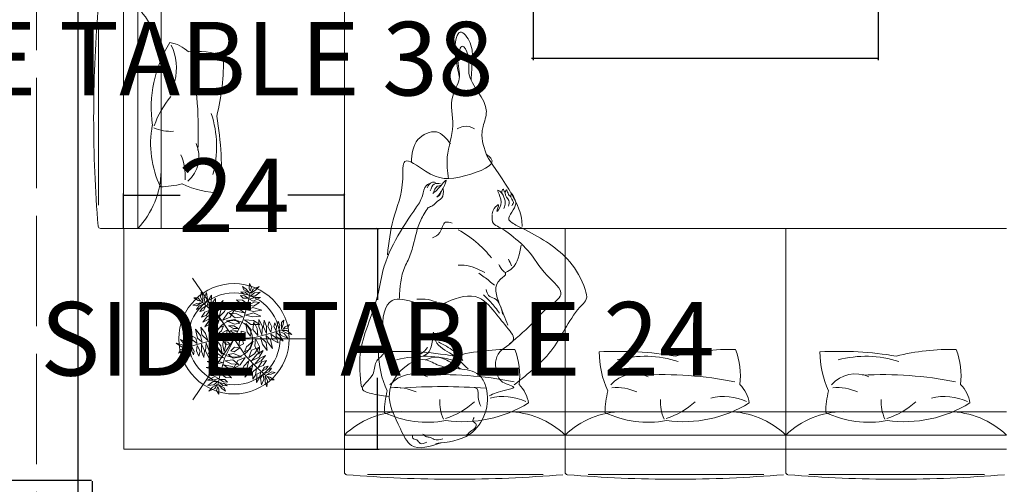
# Model space of a CAD drawing. Units: inches. Extents: x -48 to 50072, y 0 to 21068.
# Tile 48 of 75: x 16 to 123, y 687 to 738. Entities that reach past the tile are written whole.
import ezdxf

# ---------------------------------------------------------------- set-up
doc = ezdxf.new("R2010")
doc.units = ezdxf.units.IN
doc.header["$MEASUREMENT"] = 0
doc.linetypes.add('ACAD_ISO02W100', pattern=[15, 12, -3])
for name, color, linetype, lineweight in [('A-ANNO-DIMS', 2, 'Continuous', 18), ('A-ENTG', 8, 'Continuous', 13), ('C-PROP', 7, 'Continuous', 25), ('C-PROP-REF', 32, 'ACAD_ISO02W100', 13), ('FURNITURE', 44, 'Continuous', 18)]:
    doc.layers.add(name, color=color, linetype=linetype, lineweight=lineweight)
doc.styles.get("Standard").update_dxf_attribs({"font": 'arial.ttf'})
doc.dimstyles.get("Standard").update_dxf_attribs({"dimtxt": 8, "dimasz": 0.18, "dimexe": 0.18, "dimexo": 0.0625, "dimgap": 0.09, "dimtad": 0, "dimtih": 1, "dimtoh": 1, "dimdec": 1, "dimzin": 0, "dimdsep": 46, "dimlunit": 4, "dimtxsty": 'Standard', "dimblk": 'ARCHTICK', "dimcen": 0.09, "dimadec": 0, "dimazin": 0, "dimtfac": 1, "dimtdec": 1, "dimtofl": 0, "dimtmove": 0, "dimatfit": 3, "dimldrblk": 'ARCHTICK', "dimfxl": 1, "dimtolj": 1, "dimtzin": 0, "dimarcsym": 0})

# ---------------------------------------------------------------- blocks, each defined once
blk = doc.blocks.new('SIDE TABLE 2X2')
at = {"layer": 'FURNITURE'}
for q in [(622.06, 188.07), (609.55, 181.47), (622.04, 174.85)]:
    blk.add_line((617.55, 181.47), q, dxfattribs=at)
blk.add_lwpolyline([(605.55, 169.47), (629.55, 169.47), (629.55, 193.47), (605.55, 193.47)], close=True, dxfattribs=at)
for radius in [6, 5, 2]:
    blk.add_circle((617.55, 181.47), radius, dxfattribs=at)
blk = doc.blocks.new('DFGS')
at = {"layer": 'FURNITURE'}
for centre, radius, start, end in [((-6087.14, 813.36), 9.64, 104.9394, 132.5633), ((-6112.38, 805.26), 28.66, 21.6133, 37.4184), ((-6094.33, 816.04), 4.48, 81.3108, 116.3418), ((-6080.05, 821.2), 16.31, 184.0297, 223.6176), ((-6099.45, 813.66), 7.12, 22.214, 60.8038), ((-6126.91, 783.89), 49.66, 32.8076, 46.9), ((-6094.76, 804.41), 13.97, 20.7975, 53.8819), ((-6116.99, 784.16), 44.49, 32.4999, 45.375), ((-6080.96, 813.35), 11.17, 174.5959, 197.1556), ((-6092.61, 815.13), 5.43, 281.6061, 309.1892), ((-6087.9, 807.73), 4.17, 346.5527, 60.4145), ((-6080.21, 815.37), 12.85, 204.9913, 241.6537), ((-6089.91, 803.33), 6.58, 30.5945, 59.6065), ((-6086.56, 817.99), 12.2, 280.9279, 305.5545), ((-6095.16, 815.51), 14.47, 307.7029, 318.9387)]:
    blk.add_arc(centre, radius, start, end, dxfattribs=at)
blk = doc.blocks.new('3+2 seater sofa')
at = {"layer": 'FURNITURE', "ltscale": 3}
for p, q in [((1464.23, 851.06), (1464.23, 827.06)), ((1484.15, 839.06), (1484.15, 851.06)), ((1484.15, 839.06), (1484.15, 827.06)), ((1392.23, 827.06), (1416.23, 827.06)), ((1416.23, 827.06), (1440.23, 827.06)), ((1440.23, 827.06), (1464.23, 827.06)), ((1404.23, 807.13), (1392.23, 807.13)), ((1404.23, 807.13), (1416.23, 807.13)), ((1428.23, 807.13), (1416.23, 807.13)), ((1428.23, 807.13), (1440.23, 807.13)), ((1452.23, 807.13), (1440.23, 807.13)), ((1452.23, 807.13), (1464.23, 807.13))]:
    blk.add_line(p, q, dxfattribs=at)
at = {"layer": 'FURNITURE'}
for p, q in [((1486.69, 839.06), (1486.69, 851.06)), ((1488.23, 827.03, 0), (1488.23, 851.06)), ((1490.98, 848.68), (1490.98, 839.06)), ((1484.15, 844.83), (1484.15, 839.06)), ((1484.15, 833.29), (1484.15, 839.06)), ((1484.15, 839.06, 0), (1484.15, 827.06)), ((1486.69, 839.06), (1486.69, 827.06)), ((1490.98, 829.57), (1490.98, 839.06)), ((1416.23, 800.54), (1416.23, 827.06)), ((1440.23, 800.54), (1440.23, 827.06)), ((1464.23, 800.54), (1464.23, 827.06)), ((1490.74, 827.06), (1464.23, 827.06)), ((1484.13, 827.06), (1490.75, 827.06)), ((1398.46, 807.13), (1404.23, 807.13)), ((1410, 807.13), (1404.23, 807.13)), ((1404.23, 807.13, 0), (1416.23, 807.13)), ((1416.23, 807.16), (1416.23, 800.53)), ((1422.46, 807.13), (1428.23, 807.13)), ((1434, 807.13), (1428.23, 807.13)), ((1428.23, 807.13, 0), (1440.23, 807.13)), ((1440.23, 807.16), (1440.23, 800.53)), ((1446.46, 807.13), (1452.23, 807.13)), ((1458, 807.13), (1452.23, 807.13)), ((1452.23, 807.13, 0), (1464.23, 807.13)), ((1464.23, 807.16), (1464.23, 800.53)), ((1404.23, 804.59), (1392.23, 804.59)), ((1404.23, 804.59), (1416.23, 804.59)), ((1428.23, 804.59), (1416.23, 804.59)), ((1428.23, 804.59), (1440.23, 804.59)), ((1452.23, 804.59), (1440.23, 804.59)), ((1452.23, 804.59), (1464.23, 804.59)), ((1416.26, 803.06, 0), (1392.23, 803.06)), ((1440.26, 803.06, 0), (1416.23, 803.06)), ((1464.26, 803.06, 0), (1440.23, 803.06)), ((1394.6, 800.3), (1404.23, 800.3)), ((1413.72, 800.3), (1404.23, 800.3)), ((1418.6, 800.3), (1428.23, 800.3)), ((1437.72, 800.3), (1428.23, 800.3)), ((1442.6, 800.3), (1452.23, 800.3)), ((1461.72, 800.3), (1452.23, 800.3))]:
    blk.add_line(p, q, dxfattribs=at)
for centre, radius, start, end in [((1493.43, 844.68), 9.28, 136.5598, 179.0844), ((1348.3, 838.96), 143.19, 0.0378, 4.7508), ((1348.3, 839.15), 143.19, 355.2492, 359.9622), ((1493.43, 833.43), 9.28, 180.9156, 223.4402), ((1490.74, 827.31), 0.255, 270, 355.4933), ((1398.61, 797.86), 9.28, 90.9156, 133.4402), ((1409.85, 797.86), 9.28, 46.5598, 89.0844), ((1422.61, 797.86), 9.28, 90.9156, 133.4402), ((1433.85, 797.86), 9.28, 46.5598, 89.0844), ((1446.61, 797.86), 9.28, 90.9156, 133.4402), ((1457.85, 797.86), 9.28, 46.5598, 89.0844), ((1404.32, 942.98), 143.19, 265.2492, 269.9622), ((1404.13, 942.98), 143.19, 270.0378, 274.7508), ((1415.97, 800.54), 0.255, 274.5067, 0), ((1428.32, 942.98), 143.19, 265.2492, 269.9622), ((1428.13, 942.98), 143.19, 270.0378, 274.7508), ((1439.97, 800.54), 0.255, 274.5067, 0), ((1452.32, 942.98), 143.19, 265.2492, 269.9622), ((1452.13, 942.98), 143.19, 270.0378, 274.7508), ((1463.97, 800.54), 0.255, 274.5067, 0)]:
    blk.add_arc(centre, radius, start, end, dxfattribs=at)
at = {"layer": 'FURNITURE', "yscale": 0.8336162403020807, "zscale": 0.8336162403020807}
for p, xscale, rotation in [((-2239.7, -2678.91), -0.8336162403020807, 35.78436137719967), ((4922.38, 4530.98), 0.8336162403020807, 54.21563862280032), ((4946.38, 4530.98), 0.8336162403020807, 54.21563862280032), ((4970.38, 4530.98), 0.8336162403020807, 54.21563862280032)]:
    blk.add_blockref('DFGS', p, dxfattribs=dict(at, xscale=xscale, rotation=rotation))
blk = doc.blocks.new('Women')
for p, q in [((543.24, 3443.84, -275.77), (543.24, 3443.84, -275.77)), ((536.73, 3442.75, -275.77), (536.73, 3442.75, -275.77)), ((543.24, 3442.75, -275.77), (543.24, 3442.75, -275.77)), ((544.33, 3443.3, -275.77), (544.33, 3443.3, -275.77))]:
    blk.add_line(p, q)
at = {"ltscale": 3}
for centre, radius, start, end in [((540.53, 3448.44, -275.77), 1.62, 79.5148, 123.0894), ((540.33, 3447.37, -275.77), 2.71, 63.6392, 79.5148)]:
    blk.add_arc(centre, radius, start, end, dxfattribs=at)
for start, end in [(90.0228, 94.419), (85.6266, 90.0228)]:
    blk.add_arc((543.1, 3361, -303.2), 60.76, start, end)
for points, knots in [([(540, 3455.11, -275.77), (539.96, 3455.83, -275.77), (539.88, 3457.2, -275.77), (539.79, 3458.92, -275.77), (541.38, 3461.08, -275.77), (541.88, 3458.63, -275.77), (541.63, 3457.17, -275.77), (541.42, 3456.09, -275.77), (541.3, 3455.47, -275.77)], [0, 0, 0, 0, 46.697433, 88.465151, 123.324676, 161.835136, 191.877979, 232.626852, 232.626852, 232.626852, 232.626852]), ([(538.22, 3446.72, -275.77), (538.57, 3447.63, -275.77), (538.99, 3448.73, -275.77), (538.63, 3450.39, -275.77), (537.75, 3452.65, -275.77), (540.77, 3455.04, -275.77), (540.02, 3457.37, -275.77), (541.02, 3459.34, -275.77), (541.69, 3456.94, -275.77), (540.9, 3455.37, -275.77), (542.5, 3452.99, -275.77), (541.62, 3450.02, -275.77), (542.8, 3447.11, -275.77), (542.57, 3445.15, -275.77), (542.48, 3444.36, -275.77)], [0, 0, 0, 0, 60.970115, 74.178445, 111.267097, 210.963126, 255.074467, 279.515708, 307.41666, 359.287359, 403.554034, 473.492101, 549.720465, 601.59141, 601.59141, 601.59141, 601.59141]), ([(546.5, 3446.13, -275.77), (546.43, 3447.04, -275.77), (546.31, 3448.71, -275.77), (543.66, 3449.95, -275.77), (542.7, 3448.73, -275.77), (542.24, 3448.14, -275.77)], [0, 0, 0, 0, 56.575903, 104.225618, 148.354052, 148.354052, 148.354052, 148.354052]), ([(534.44, 3439.16, -275.77), (534.48, 3439.74, -275.77), (534.64, 3442.24, -275.77), (539.62, 3448.28, -275.77), (537.06, 3445.84, -275.77), (541.78, 3444.17, -275.77), (544.01, 3444.26, -275.77), (547.6, 3447.18, -275.77), (547.23, 3443, -275.77), (548.63, 3440.29, -275.77), (548.95, 3437.41, -275.77), (549.1, 3436.09, -275.77)], [0, 0, 0, 0, 42.167956, 184.846032, 188.510605, 261.118314, 357.582537, 412.070511, 453.838275, 554.467695, 638.871943, 638.871943, 638.871943, 638.871943]), ([(543.72, 3442.36, -275.77), (543.51, 3442.61, -275.77), (543.15, 3443.06, -275.77), (542.48, 3444.55, -275.77), (543.22, 3443.72, -275.77), (543.57, 3443.25, -275.77), (543.96, 3442.94, -275.77), (544.17, 3442.76, -275.77)], [0, 0, 0, 0, 25.892768, 46.183307, 59.392839, 73.451861, 90.844376, 90.844376, 90.844376, 90.844376]), ([(544.44, 3443.03, -275.77), (544.34, 3443.34, -275.77), (544.17, 3443.92, -275.77), (543.58, 3443.85, -275.77), (543.32, 3443.82, -275.77)], [0, 0, 0, 0, 18.54008, 34.34859, 34.34859, 34.34859, 34.34859]), ([(544.09, 3442.81, -275.77), (544.04, 3443, -275.77), (543.96, 3443.29, -275.77), (543.74, 3443.48, -275.77), (543.68, 3443.54, -275.77)], [0, 0, 0, 0, 12.899473, 18.839157, 18.839157, 18.839157, 18.839157]), ([(544.78, 3443.38, -275.77), (544.64, 3443.64, -275.77), (544.43, 3444.03, -275.77), (544.02, 3443.98, -275.77), (543.88, 3443.96, -275.77)], [0, 0, 0, 0, 16.968689, 25.728505, 25.728505, 25.728505, 25.728505]), ([(545.63, 3441.73, -275.77), (545.51, 3441.98, -275.77), (545.23, 3442.59, -275.77), (545.09, 3443.61, -275.77), (544.49, 3443.87, -275.77), (544.28, 3443.96, -275.77)], [0, 0, 0, 0, 18.740722, 44.970985, 59.745283, 59.745283, 59.745283, 59.745283]), ([(534.98, 3439.25, -275.77), (535.18, 3439.35, -275.77), (535.5, 3439.52, -275.77), (536.1, 3439.99, -275.77), (535.52, 3440.79, -275.77), (534.94, 3441.7, -275.77), (535.37, 3442.42, -275.77), (535.62, 3442.83, -275.77)], [0, 0, 0, 0, 14.897426, 24.638003, 44.249327, 65.81281, 94.158391, 94.158391, 94.158391, 94.158391]), ([(535.62, 3442.83, -275.77), (535.68, 3442.61, -275.77), (535.76, 3442.25, -275.77), (535.3, 3441.87, -275.77), (535.47, 3441.58, -275.77), (535.57, 3441.42, -275.77)], [0, 0, 0, 0, 13.770952, 22.047872, 32.93541, 32.93541, 32.93541, 32.93541]), ([(535.94, 3441.37, -275.77), (535.88, 3441.59, -275.77), (535.73, 3442.14, -275.77), (536.5, 3442.52, -275.77), (536.12, 3443.33, -275.77), (536, 3442.68, -275.77), (535.8, 3442.49, -275.77), (535.69, 3442.39, -275.77)], [0, 0, 0, 0, 13.81853, 34.349896, 42.048978, 50.626809, 61.603847, 61.603847, 61.603847, 61.603847]), ([(537.72, 3440.56, -275.77), (537.68, 3440.74, -275.77), (537.61, 3441.1, -275.77), (536.74, 3441.86, -275.77), (537.48, 3440.4, -275.77), (536.19, 3441.86, -275.77), (537.47, 3443.4, -275.77), (536.74, 3442.92, -275.77), (536.46, 3442.5, -275.77), (536.22, 3441.82, -275.77), (536.37, 3441.34, -275.77), (536.43, 3441.13, -275.77)], [0, 0, 0, 0, 13.622009, 27.045047, 42.301032, 59.74223, 94.71225, 98.491569, 110.440566, 128.701216, 142.844466, 142.844466, 142.844466, 142.844466]), ([(536.38, 3442.9, -275.77), (536.42, 3443.07, -275.77), (536.51, 3443.43, -275.77), (536.75, 3442.89, -275.77), (536.62, 3442.75, -275.77), (536.58, 3442.71, -275.77)], [0, 0, 0, 0, 7.980072, 16.932683, 20.710806, 20.710806, 20.710806, 20.710806]), ([(544.68, 3441.23, -275.77), (544.5, 3441.29, -275.77), (544.1, 3441.43, -275.77), (543.66, 3441.99, -275.77), (542.92, 3442.25, -275.77), (543.07, 3443.67, -275.77), (543.28, 3442.74, -275.77), (543.51, 3442.48, -275.77), (543.65, 3442.4, -275.77), (543.72, 3442.36, -275.77)], [0, 0, 0, 0, 12.228513, 27.193094, 45.006155, 62.152179, 75.922416, 81.425571, 86.507745, 86.507745, 86.507745, 86.507745]), ([(547.8, 3431.37, -275.77), (547.74, 3432.56, -275.77), (547.67, 3434.02, -275.77), (546.69, 3435.75, -275.77), (546.17, 3437.46, -275.77), (545.78, 3439.51, -275.77), (544.97, 3440.78, -275.77), (544.68, 3441.23, -275.77)], [0, 0, 0, 0, 76.228588, 93.60718, 130.36676, 193.495034, 228.582316, 228.582316, 228.582316, 228.582316]), ([(551.94, 3421.7, -275.77), (552.07, 3422.91, -275.77), (552.43, 3426.3, -275.77), (550.26, 3430.29, -275.77), (549.45, 3436.2, -275.77), (547.26, 3439.37, -275.77), (545.63, 3441.73, -275.77)], [0, 0, 0, 0, 78.836785, 220.670789, 284.620897, 468.343596, 468.343596, 468.343596, 468.343596]), ([(535.98, 3438.49, -275.77), (536.29, 3438.7, -275.77), (536.8, 3439.05, -275.77), (537.77, 3439.46, -275.77), (537.74, 3440.1, -275.77), (537.72, 3440.48, -275.77)], [0, 0, 0, 0, 25.616728, 40.995926, 63.070156, 63.070156, 63.070156, 63.070156]), ([(535.33, 3421.95, -275.77), (533.78, 3423.17, -275.77), (530.71, 3425.6, -275.77), (529.22, 3429.43, -275.77), (527.29, 3431.3, -275.77), (527.83, 3433.19, -275.77), (529.49, 3436.17, -275.77), (532.62, 3438.08, -275.77), (534.69, 3439.1, -275.77), (534.98, 3439.25, -275.77)], [0, 0, 0, 0, 126.89883, 252.166699, 268.447012, 291.91585, 367.798424, 497.771558, 519.675303, 519.675303, 519.675303, 519.675303]), ([(542.05, 3439.54, -275.77), (542.32, 3439.62, -275.77), (543.07, 3439.84, -275.77), (543.21, 3438.4, -275.77), (543.92, 3438.08, -275.77), (544.22, 3437.94, -275.77)], [0, 0, 0, 0, 15.981012, 44.422669, 65.960047, 65.960047, 65.960047, 65.960047]), ([(535.83, 3426.41, -275.77), (534.87, 3427.22, -275.77), (533.32, 3428.53, -275.77), (531.8, 3430.39, -275.77), (529.44, 3431.88, -275.77), (532.32, 3434.11, -275.77), (533.51, 3436.52, -275.77), (535.21, 3437.87, -275.77), (535.98, 3438.49, -275.77)], [0, 0, 0, 0, 80.80909, 130.775511, 169.211303, 225.758914, 301.315819, 364.276194, 364.276194, 364.276194, 364.276194]), ([(537.78, 3435.77, -275.77), (538.25, 3436.3, -275.77), (539.29, 3437.5, -275.77), (540.65, 3438.35, -275.77), (541.41, 3438.82, -275.77)], [0, 0, 0, 0, 46.172455, 104.424665, 104.424665, 104.424665, 104.424665]), ([(536.25, 3434.16, -275.77), (536, 3434.3, -275.77), (534.95, 3434.9, -275.77), (534.73, 3436.17, -275.77), (534.56, 3437.13, -275.77)], [0, 0, 0, 0, 19.085058, 77.715078, 77.715078, 77.715078, 77.715078]), ([(536.01, 3428.45, -275.77), (536.3, 3429.16, -275.77), (536.9, 3430.69, -275.77), (537.79, 3433.01, -275.77), (536.01, 3433.96, -275.77), (536.57, 3434.35, -275.77), (536.8, 3434.66, -275.77), (536.93, 3434.93, -275.77), (536.98, 3435.04, -275.77)], [0, 0, 0, 0, 53.059535, 113.04795, 131.800676, 139.285566, 150.580969, 158.469393, 158.469393, 158.469393, 158.469393]), ([(538.51, 3434.16, -275.77), (539.24, 3434.53, -275.77), (540.17, 3435, -275.77), (541.19, 3434.97, -275.77), (541.41, 3434.96, -275.77)], [0, 0, 0, 0, 52.46729, 66.585747, 66.585747, 66.585747, 66.585747]), ([(537.46, 3432.79, -275.77), (537.83, 3433.09, -275.77), (538.38, 3433.54, -275.77), (538.96, 3433.94, -275.77), (539.15, 3434.08, -275.77)], [0, 0, 0, 0, 31.413427, 46.591217, 46.591217, 46.591217, 46.591217]), ([(538.05, 3420.77, -275.77), (537.55, 3420.97, -275.77), (536.8, 3421.27, -275.77), (534.75, 3421.69, -275.77), (536.78, 3422.1, -275.77), (537.38, 3423.51, -275.77), (537.53, 3425.74, -275.77), (534.92, 3426.61, -275.77), (536.1, 3428.28, -275.77), (537.28, 3429.57, -275.77), (539.14, 3432.15, -275.77), (542.1, 3431.31, -275.77), (543.83, 3430.28, -275.77), (544.68, 3430.34, -275.77), (544.99, 3430.36, -275.77)], [0, 0, 0, 0, 40.880348, 61.700866, 91.143691, 114.873082, 167.923204, 214.466852, 232.950995, 283.095365, 341.741032, 417.680752, 453.135852, 472.889302, 472.889302, 472.889302, 472.889302]), ([(536.58, 3429.65, -275.77), (536.74, 3430.35, -275.77), (536.95, 3431.31, -275.77), (538.21, 3431.56, -275.77), (538.3, 3432.06, -275.77), (538.35, 3432.31, -275.77)], [0, 0, 0, 0, 41.814842, 57.597678, 72.667081, 72.667081, 72.667081, 72.667081]), ([(536.9, 3429.73, -275.77), (537.21, 3430.15, -275.77), (537.75, 3430.86, -275.77), (538.39, 3431.48, -275.77), (538.67, 3431.74, -275.77)], [0, 0, 0, 0, 33.886621, 58.836239, 58.836239, 58.836239, 58.836239]), ([(543.78, 3430.96, -275.77), (544.18, 3431.09, -275.77), (544.87, 3431.31, -275.77), (545.58, 3431.27, -275.77), (545.89, 3431.26, -275.77)], [0, 0, 0, 0, 27.147531, 46.900981, 46.900981, 46.900981, 46.900981]), ([(548.92, 3420.68, -275.77), (549.46, 3420.74, -275.77), (550.37, 3420.84, -275.77), (552.58, 3421.47, -275.77), (550.35, 3422.84, -275.77), (550.61, 3424.44, -275.77), (548.99, 3425.54, -275.77), (549.94, 3428.03, -275.77), (549.25, 3431.84, -275.77), (546.97, 3431.16, -275.77), (545.99, 3430.87, -275.77)], [0, 0, 0, 0, 39.625932, 66.399645, 109.367011, 140.345835, 165.401676, 219.739472, 296.252236, 353.603905, 353.603905, 353.603905, 353.603905]), ([(540.34, 3423.68, -275.77), (540.97, 3424.31, -275.77), (542.15, 3425.48, -275.77), (543.96, 3426.26, -275.77), (544.15, 3428.35, -275.77), (544.12, 3425.3, -275.77), (545.28, 3425.04, -275.77), (545.82, 3424.93, -275.77)], [0, 0, 0, 0, 58.393088, 109.526114, 121.740606, 162.697201, 197.973392, 197.973392, 197.973392, 197.973392]), ([(540.89, 3424.6, -275.77), (541.21, 3424.95, -275.77), (541.96, 3425.79, -275.77), (542.97, 3426.31, -275.77), (543.54, 3426.61, -275.77)], [0, 0, 0, 0, 31.248067, 73.627741, 73.627741, 73.627741, 73.627741]), ([(545.47, 3425.33, -275.77), (545.27, 3425.47, -275.77), (544.97, 3425.67, -275.77), (544.79, 3425.97, -275.77), (544.74, 3426.06, -275.77)], [0, 0, 0, 0, 15.689416, 22.930946, 22.930946, 22.930946, 22.930946]), ([(543.84, 3415.58, -275.77), (542.51, 3415.72, -275.77), (540.18, 3415.98, -275.77), (538.21, 3418.8, -275.77), (538.1, 3421.2, -275.77), (539.38, 3424.07, -275.77), (542.66, 3423.34, -275.77), (545.34, 3425.15, -275.77), (547.88, 3423.7, -275.77), (549.47, 3420.6, -275.77), (547.97, 3417.84, -275.77), (546.52, 3414.58, -275.77), (544.48, 3415.25, -275.77), (543.26, 3415.65, -275.77)], [0, 0, 0, 0, 83.935274, 146.390702, 207.043537, 236.474222, 338.687878, 374.142978, 438.985032, 497.846364, 587.349285, 634.808067, 705.826625, 705.826625, 705.826625, 705.826625]), ([(541.16, 3423.68, -275.77), (541.64, 3424.02, -275.77), (542.42, 3424.57, -275.77), (543.77, 3425.12, -275.77), (544.55, 3424.83, -275.77), (544.96, 3424.67, -275.77)], [0, 0, 0, 0, 38.642267, 63.395223, 91.234873, 91.234873, 91.234873, 91.234873]), ([(538.93, 3419.63, -275.77), (539.08, 3419.94, -275.77), (539.35, 3420.53, -275.77), (539.14, 3421.37, -275.77), (539.51, 3421.66, -275.77), (539.63, 3421.65, -275.77), (539.67, 3421.65, -275.77)], [0, 0, 0, 0, 22.483571, 42.779574, 47.617419, 50.301561, 50.301561, 50.301561, 50.301561]), ([(540.46, 3416.51, -275.77), (540.29, 3416.68, -275.77), (540, 3416.97, -275.77), (539.51, 3417.23, -275.77), (539.36, 3417.78, -275.77), (539.94, 3417.94, -275.77), (539.76, 3418.24, -275.77), (539.67, 3418.41, -275.77)], [0, 0, 0, 0, 16.156044, 26.634965, 36.11877, 44.709969, 54.474279, 54.474279, 54.474279, 54.474279]), ([(543.09, 3416.08, -275.77), (543.41, 3416, -275.77), (543.94, 3415.86, -275.77), (544.46, 3416.32, -275.77), (544.93, 3416.25, -275.77), (545.07, 3416.5, -275.77), (545.19, 3416.55, -275.77), (545.24, 3416.57, -275.77)], [0, 0, 0, 0, 20.1757, 33.392446, 41.555809, 47.247785, 50.24837, 50.24837, 50.24837, 50.24837]), ([(544.81, 3415.71, -275.77), (545.08, 3415.6, -275.77), (545.55, 3415.39, -275.77), (545.82, 3416.04, -275.77), (546.43, 3416.04, -275.77), (546.37, 3416.37, -275.77), (546.34, 3416.51, -275.77)], [0, 0, 0, 0, 16.326725, 27.710838, 37.931003, 45.977913, 45.977913, 45.977913, 45.977913])]:
    blk.add_open_spline(points, degree=3, knots=knots, dxfattribs=at)
for points in [[(543.68, 3443.54, -275.77), (543.53, 3443.58, -275.77), (543.39, 3443.62, -275.77), (543.24, 3443.65, -275.77)], [(535.61, 3434.88, -275.77), (535.72, 3435.12, -275.77), (535.83, 3435.36, -275.77), (535.93, 3435.6, -275.77)]]:
    blk.add_open_spline(points, degree=3, dxfattribs=at)
blk = doc.blocks.new('A$C27D05267')
for p, q in [((2.677, 4.042), (2.671, 3.86)), ((2.752, 3.911), (2.677, 4.042)), ((0.92, 3.773), (0.893, 3.54)), ((0.974, 3.592), (0.92, 3.773)), ((1.029, 3.507), (1.114, 3.71)), ((1.114, 3.71), (1.148, 3.46)), ((1.185, 3.438), (1.287, 3.619)), ((1.287, 3.619), (1.276, 3.317)), ((2.481, 3.65), (2.364, 3.743)), ((2.364, 3.743), (2.522, 3.728)), ((2.47, 3.818), (2.429, 3.938)), ((2.429, 3.938), (2.56, 3.843)), ((2.667, 3.707), (2.47, 3.818)), ((2.637, 3.633), (2.481, 3.65)), ((2.522, 3.728), (2.637, 3.633)), ((2.56, 3.843), (2.667, 3.707)), ((2.62, 3.299), (2.71, 3.732)), ((2.671, 3.86), (2.706, 3.76)), ((2.706, 3.76), (2.752, 3.911)), ((2.708, 3.587), (2.859, 3.705)), ((2.82, 3.839), (2.727, 3.692)), ((2.727, 3.692), (2.905, 3.795)), ((3.035, 3.933), (2.82, 3.839)), ((2.859, 3.705), (3.077, 3.733)), ((3.077, 3.733), (2.878, 3.579)), ((2.905, 3.795), (3.035, 3.933)), ((0.612, 3.251), (0.759, 3.317)), ((0.737, 3.226), (0.612, 3.251)), ((0.646, 3.518), (0.801, 3.421)), ((0.797, 3.518), (0.646, 3.518)), ((0.931, 3.342), (0.737, 3.226)), ((0.759, 3.317), (0.931, 3.342)), ((0.904, 3.402), (0.797, 3.518)), ((0.801, 3.421), (0.904, 3.402)), ((0.84, 3.226), (0.98, 3.279)), ((0.98, 3.279), (0.888, 3.152)), ((0.893, 3.54), (0.974, 3.386)), ((1.261, 3.097), (0.931, 3.391)), ((0.974, 3.386), (0.974, 3.592)), ((1.055, 3.317), (1.029, 3.507)), ((1.148, 3.46), (1.055, 3.317)), ((1.136, 3.237), (1.185, 3.438)), ((1.276, 3.317), (1.136, 3.237)), ((1.299, 3.103), (1.325, 3.353)), ((1.325, 3.353), (1.432, 3.496)), ((1.432, 3.496), (1.438, 3.237)), ((1.47, 3.193), (1.719, 3.421)), ((1.719, 3.421), (1.606, 3.136)), ((1.649, 3.108), (1.881, 3.284)), ((1.881, 3.284), (1.762, 3.017)), ((2.273, 3.181), (2.074, 3.321)), ((2.074, 3.321), (2.319, 3.282)), ((2.342, 3.326), (2.21, 3.45)), ((2.21, 3.45), (2.421, 3.435)), ((2.319, 3.282), (2.545, 3.144)), ((2.585, 3.311), (2.342, 3.326)), ((2.454, 3.504), (2.354, 3.601)), ((2.354, 3.601), (2.497, 3.589)), ((2.421, 3.435), (2.585, 3.311)), ((2.453, 2.71), (2.62, 3.299)), ((2.631, 3.506), (2.454, 3.504)), ((2.497, 3.589), (2.631, 3.506)), ((2.644, 3.269), (2.874, 3.371)), ((2.83, 3.216), (2.644, 3.269)), ((2.679, 3.477), (2.878, 3.535)), ((2.818, 3.396), (2.679, 3.477)), ((2.878, 3.579), (2.708, 3.587)), ((3.086, 3.537), (2.818, 3.396)), ((3.051, 3.35), (2.83, 3.216)), ((2.874, 3.371), (3.051, 3.35)), ((2.878, 3.535), (3.086, 3.537)), ((0.748, 3.097), (0.84, 3.226)), ((0.888, 3.152), (0.748, 3.097)), ((0.867, 3.017), (0.948, 3.136)), ((1.001, 3.056), (0.867, 3.017)), ((0.925, 2.817), (1.044, 2.993)), ((0.948, 3.136), (1.087, 3.21)), ((1.087, 3.21), (1.001, 3.056)), ((1.044, 2.993), (1.233, 3.072)), ((1.233, 3.072), (1.099, 2.869)), ((1.125, 2.828), (1.357, 2.954)), ((1.357, 2.954), (1.189, 2.737)), ((1.687, 2.657), (1.261, 3.097)), ((1.438, 3.237), (1.299, 3.103)), ((1.432, 2.965), (1.47, 3.193)), ((1.606, 3.136), (1.432, 2.965)), ((1.578, 2.822), (1.649, 3.108)), ((1.762, 3.017), (1.578, 2.822)), ((1.708, 2.699), (1.891, 2.971)), ((1.891, 2.971), (2.14, 3.103)), ((2.215, 2.941), (1.939, 2.962)), ((1.939, 2.962), (2.159, 2.785)), ((2.24, 3.149), (1.958, 3.161)), ((1.958, 3.161), (2.18, 3.034)), ((2.14, 3.103), (1.972, 2.817)), ((2.18, 3.034), (2.497, 2.973)), ((2.443, 2.831), (2.215, 2.941)), ((2.497, 2.973), (2.24, 3.149)), ((2.545, 3.144), (2.273, 3.181)), ((2.541, 2.887), (2.824, 2.968)), ((2.802, 2.825), (2.541, 2.887)), ((2.592, 3.085), (2.808, 3.166)), ((2.826, 3.02), (2.592, 3.085)), ((2.808, 3.166), (3.13, 3.064)), ((2.824, 2.968), (3.092, 2.855)), ((3.13, 3.064), (2.826, 3.02)), ((1.099, 2.869), (0.925, 2.817)), ((0.969, 2.635), (1.125, 2.828)), ((1.189, 2.737), (0.969, 2.635)), ((1.201, 2.693), (1.05, 2.454)), ((1.05, 2.454), (1.27, 2.583)), ((1.181, 2.301), (1.191, 2.583)), ((1.191, 2.583), (1.354, 2.294)), ((1.482, 2.828), (1.201, 2.693)), ((1.368, 2.567), (1.212, 2.339)), ((1.27, 2.583), (1.482, 2.828)), ((1.578, 2.71), (1.368, 2.567)), ((1.476, 2.44), (1.578, 2.71)), ((2.116, 2.021), (1.687, 2.657)), ((1.972, 2.817), (1.708, 2.699)), ((2.143, 2.725), (1.841, 2.675)), ((1.841, 2.675), (2.139, 2.562)), ((2.116, 2.021), (2.453, 2.71)), ((2.139, 2.562), (2.33, 2.592)), ((2.33, 2.592), (2.143, 2.725)), ((2.159, 2.785), (2.443, 2.831)), ((2.499, 2.713), (2.826, 2.691)), ((2.733, 2.543), (2.499, 2.713)), ((2.739, 2.35), (2.545, 2.586)), ((2.545, 2.586), (2.595, 2.271)), ((3.064, 2.541), (2.733, 2.543)), ((2.843, 2.645), (2.799, 2.365)), ((3.092, 2.855), (2.802, 2.825)), ((2.826, 2.691), (3.064, 2.541)), ((2.962, 2.395), (2.843, 2.645)), ((3.155, 2.477), (3.024, 2.727)), ((3.024, 2.727), (3.025, 2.472)), ((3.199, 2.465), (3.221, 2.707)), ((3.221, 2.707), (3.31, 2.475)), ((3.358, 2.477), (3.4, 2.654)), ((3.4, 2.654), (3.493, 2.463)), ((3.569, 2.469), (3.603, 2.604)), ((3.603, 2.604), (3.665, 2.475)), ((3.709, 2.519), (3.731, 2.667)), ((3.731, 2.667), (3.797, 2.522)), ((3.797, 2.522), (3.772, 2.376)), ((3.849, 2.612), (3.933, 2.708)), ((3.852, 2.386), (3.849, 2.612)), ((3.916, 2.547), (3.852, 2.386)), ((3.933, 2.708), (3.916, 2.547)), ((4.146, 2.545), (3.986, 2.459)), ((4.071, 2.414), (4.146, 2.545)), ((0.567, 2.002), (0.497, 2.167)), ((0.497, 2.167), (0.723, 2.042)), ((0.777, 2.048), (0.704, 2.378)), ((0.704, 2.378), (0.895, 2.137)), ((0.941, 2.161), (0.904, 2.45)), ((0.904, 2.45), (1.076, 2.213)), ((1.076, 2.213), (1.153, 1.956)), ((1.325, 2.007), (1.181, 2.301)), ((1.212, 2.339), (1.476, 2.44)), ((1.354, 2.294), (1.325, 2.007)), ((1.519, 2.396), (1.412, 2.111)), ((1.412, 2.111), (1.659, 2.311)), ((1.729, 2.493), (1.519, 2.396)), ((1.659, 2.311), (1.729, 2.493)), ((1.864, 2.339), (1.702, 2.253)), ((1.702, 2.253), (1.74, 2.1)), ((1.74, 2.1), (1.838, 2.163)), ((1.838, 2.163), (1.864, 2.339)), ((2.11, 2.495), (1.909, 2.493)), ((1.909, 2.493), (2.1, 2.401)), ((2.076, 2.344), (1.974, 2.314)), ((1.974, 2.314), (2.076, 2.253)), ((2.226, 2.3), (2.076, 2.344)), ((2.076, 2.253), (2.226, 2.3)), ((2.1, 2.401), (2.265, 2.397)), ((2.265, 2.397), (2.11, 2.495)), ((2.524, 2.263), (2.371, 2.307)), ((2.371, 2.307), (2.377, 2.19)), ((2.377, 2.19), (2.516, 2.08)), ((2.516, 2.08), (2.524, 2.263)), ((2.595, 2.271), (2.717, 2.12)), ((2.717, 2.12), (2.739, 2.35)), ((2.799, 2.365), (2.981, 2.142)), ((2.881, 2.074), (3.475, 2.223)), ((2.981, 2.142), (2.962, 2.395)), ((3.025, 2.472), (3.131, 2.167)), ((3.131, 2.167), (3.155, 2.477)), ((3.303, 2.211), (3.199, 2.465)), ((3.31, 2.475), (3.303, 2.211)), ((3.468, 2.26), (3.358, 2.477)), ((3.461, 2.188), (3.664, 2.04)), ((3.508, 1.999), (3.461, 2.188)), ((3.493, 2.463), (3.468, 2.26)), ((3.475, 2.223), (3.895, 2.362)), ((3.659, 2.317), (3.569, 2.469)), ((3.658, 2.1), (3.659, 2.261)), ((3.665, 2.475), (3.659, 2.317)), ((3.659, 2.261), (3.808, 2.118)), ((3.772, 2.376), (3.709, 2.519)), ((3.768, 2.291), (3.946, 2.219)), ((3.846, 2.14), (3.768, 2.291)), ((3.868, 2.327), (4.047, 2.224)), ((4.042, 2.32), (3.868, 2.327)), ((3.986, 2.459), (3.917, 2.379)), ((3.917, 2.379), (4.071, 2.414)), ((3.946, 2.219), (4.079, 2.044)), ((4.231, 2.18), (4.042, 2.32)), ((4.047, 2.224), (4.231, 2.18)), ((0.184, 1.818), (0, 1.861)), ((0, 1.861), (0.189, 1.722)), ((0.286, 1.823), (0.152, 1.998)), ((0.152, 1.998), (0.385, 1.902)), ((0.363, 1.715), (0.184, 1.818)), ((0.463, 1.751), (0.286, 1.823)), ((0.423, 1.924), (0.317, 2.103)), ((0.317, 2.103), (0.573, 1.942)), ((0.756, 1.819), (0.336, 1.68)), ((0.385, 1.902), (0.463, 1.751)), ((0.573, 1.781), (0.423, 1.924)), ((0.77, 1.854), (0.567, 2.002)), ((0.573, 1.942), (0.573, 1.781)), ((0.723, 2.042), (0.77, 1.854)), ((1.35, 1.968), (0.756, 1.819)), ((0.956, 1.902), (0.777, 2.048)), ((0.895, 2.137), (0.956, 1.902)), ((0.922, 1.567), (0.928, 1.831)), ((0.928, 1.831), (1.032, 1.577)), ((1.153, 1.956), (0.941, 2.161)), ((1.1, 1.875), (1.076, 1.565)), ((1.206, 1.57), (1.1, 1.875)), ((1.25, 1.899), (1.269, 1.647)), ((1.432, 1.677), (1.25, 1.899)), ((2.116, 2.021), (1.35, 1.968)), ((1.514, 1.922), (1.492, 1.692)), ((1.636, 1.77), (1.514, 1.922)), ((1.715, 1.962), (1.707, 1.779)), ((1.818, 1.783), (1.715, 1.962)), ((2.116, 2.021), (1.779, 1.332)), ((1.888, 1.897), (1.785, 1.922)), ((1.785, 1.922), (1.842, 1.819)), ((1.842, 1.819), (1.996, 1.783)), ((1.996, 1.783), (1.888, 1.897)), ((2.116, 2.021), (2.881, 2.074)), ((2.116, 2.021), (2.544, 1.384)), ((2.322, 1.934), (2.295, 1.758)), ((2.295, 1.758), (2.457, 1.843)), ((2.42, 1.997), (2.322, 1.934)), ((2.457, 1.843), (2.42, 1.997)), ((2.819, 1.931), (2.572, 1.731)), ((2.712, 1.645), (2.819, 1.931)), ((2.877, 1.747), (2.906, 2.035)), ((2.906, 2.035), (3.051, 1.741)), ((3.079, 2.086), (3.29, 1.881)), ((3.155, 1.828), (3.079, 2.086)), ((3.327, 1.592), (3.155, 1.828)), ((3.275, 2.14), (3.454, 1.994)), ((3.336, 1.905), (3.275, 2.14)), ((3.29, 1.881), (3.327, 1.592)), ((3.527, 1.664), (3.336, 1.905)), ((3.454, 1.994), (3.527, 1.664)), ((3.734, 1.875), (3.508, 1.999)), ((3.914, 1.939), (3.658, 2.1)), ((3.664, 2.04), (3.734, 1.875)), ((3.808, 2.118), (3.914, 1.939)), ((4.079, 2.044), (3.846, 2.14)), ((0.16, 1.627), (0.085, 1.497)), ((0.085, 1.497), (0.245, 1.583)), ((0.314, 1.663), (0.16, 1.627)), ((0.189, 1.722), (0.363, 1.715)), ((0.245, 1.583), (0.314, 1.663)), ((0.299, 1.334), (0.315, 1.494)), ((0.315, 1.494), (0.379, 1.655)), ((0.379, 1.655), (0.382, 1.429)), ((0.434, 1.519), (0.459, 1.666)), ((0.5, 1.375), (0.434, 1.519)), ((0.459, 1.666), (0.522, 1.523)), ((0.522, 1.523), (0.5, 1.375)), ((0.566, 1.567), (0.572, 1.725)), ((0.628, 1.438), (0.566, 1.567)), ((0.572, 1.725), (0.662, 1.573)), ((0.662, 1.573), (0.628, 1.438)), ((0.738, 1.579), (0.763, 1.782)), ((0.831, 1.388), (0.738, 1.579)), ((0.763, 1.782), (0.873, 1.564)), ((0.873, 1.564), (0.831, 1.388)), ((1.01, 1.335), (0.922, 1.567)), ((1.032, 1.577), (1.01, 1.335)), ((1.076, 1.565), (1.207, 1.314)), ((1.405, 1.351), (1.167, 1.501)), ((1.167, 1.501), (1.498, 1.498)), ((1.207, 1.314), (1.206, 1.57)), ((1.269, 1.647), (1.389, 1.397)), ((1.389, 1.397), (1.432, 1.677)), ((1.492, 1.692), (1.686, 1.456)), ((1.498, 1.498), (1.732, 1.329)), ((1.686, 1.456), (1.636, 1.77)), ((1.707, 1.779), (1.758, 1.562)), ((1.758, 1.562), (1.818, 1.783)), ((2.093, 1.48), (1.901, 1.45)), ((1.901, 1.45), (2.089, 1.317)), ((2.132, 1.71), (2.004, 1.584)), ((2.004, 1.584), (2.121, 1.547)), ((2.39, 1.367), (2.093, 1.48)), ((2.121, 1.547), (2.33, 1.686)), ((2.33, 1.686), (2.132, 1.71)), ((2.572, 1.731), (2.503, 1.549)), ((2.503, 1.549), (2.712, 1.645)), ((2.755, 1.601), (2.653, 1.332)), ((2.653, 1.332), (2.863, 1.475)), ((2.961, 1.459), (2.75, 1.214)), ((3.019, 1.703), (2.755, 1.601)), ((2.863, 1.475), (3.019, 1.703)), ((3.04, 1.459), (2.877, 1.747)), ((3.181, 1.588), (2.961, 1.459)), ((3.031, 1.349), (3.181, 1.588)), ((3.051, 1.741), (3.04, 1.459)), ((0.382, 1.429), (0.299, 1.334)), ((1.139, 1.186), (1.429, 1.217)), ((1.407, 1.074), (1.139, 1.186)), ((1.732, 1.329), (1.405, 1.351)), ((1.69, 1.154), (1.407, 1.074)), ((1.429, 1.217), (1.69, 1.154)), ((1.779, 1.332), (1.611, 0.743)), ((2.072, 1.257), (1.788, 1.211)), ((1.788, 1.211), (2.016, 1.101)), ((2.016, 1.101), (2.292, 1.079)), ((2.292, 1.079), (2.072, 1.257)), ((2.089, 1.317), (2.39, 1.367)), ((2.091, 0.939), (2.259, 1.225)), ((2.259, 1.225), (2.523, 1.343)), ((2.523, 1.343), (2.34, 1.071)), ((2.469, 1.024), (2.653, 1.219)), ((2.544, 1.384), (2.97, 0.945)), ((2.653, 1.219), (2.582, 0.934)), ((2.75, 1.214), (3.031, 1.349)), ((2.874, 1.088), (3.042, 1.305)), ((3.106, 1.214), (2.874, 1.088)), ((2.998, 0.969), (3.132, 1.173)), ((3.042, 1.305), (3.262, 1.406)), ((3.262, 1.406), (3.106, 1.214)), ((3.132, 1.173), (3.306, 1.225)), ((3.306, 1.225), (3.187, 1.049)), ((1.101, 0.977), (1.405, 1.022)), ((1.423, 0.876), (1.101, 0.977)), ((1.18, 0.692), (1.401, 0.826)), ((1.587, 0.773), (1.357, 0.67)), ((1.401, 0.826), (1.587, 0.773)), ((1.405, 1.022), (1.639, 0.957)), ((1.639, 0.957), (1.423, 0.876)), ((1.611, 0.743), (1.521, 0.31)), ((1.646, 0.73), (1.889, 0.716)), ((1.81, 0.607), (1.646, 0.73)), ((1.686, 0.897), (1.958, 0.861)), ((1.912, 0.76), (1.686, 0.897)), ((1.734, 1.068), (1.991, 0.892)), ((2.051, 1.008), (1.734, 1.068)), ((2.157, 0.72), (1.912, 0.76)), ((1.958, 0.861), (2.157, 0.72)), ((1.991, 0.892), (2.273, 0.881)), ((2.273, 0.881), (2.051, 1.008)), ((2.34, 1.071), (2.091, 0.939)), ((2.35, 0.758), (2.469, 1.024)), ((2.582, 0.934), (2.35, 0.758)), ((2.512, 0.62), (2.625, 0.906)), ((2.761, 0.848), (2.512, 0.62)), ((2.625, 0.906), (2.799, 1.077)), ((2.799, 1.077), (2.761, 0.848)), ((2.793, 0.804), (2.932, 0.939)), ((2.799, 0.546), (2.793, 0.804)), ((2.932, 0.939), (2.906, 0.689)), ((2.944, 0.422), (2.955, 0.725)), ((2.955, 0.725), (3.095, 0.804)), ((2.97, 0.945), (3.3, 0.651)), ((3.187, 1.049), (2.998, 0.969)), ((3.095, 0.804), (3.046, 0.604)), ((3.083, 0.582), (3.176, 0.725)), ((3.144, 0.832), (3.23, 0.986)), ((3.283, 0.906), (3.144, 0.832)), ((3.176, 0.725), (3.202, 0.535)), ((3.23, 0.986), (3.364, 1.024)), ((3.251, 0.763), (3.344, 0.89)), ((3.391, 0.815), (3.251, 0.763)), ((3.364, 1.024), (3.283, 0.906)), ((3.3, 0.7), (3.494, 0.815)), ((3.472, 0.725), (3.3, 0.7)), ((3.344, 0.89), (3.483, 0.945)), ((3.483, 0.945), (3.391, 0.815)), ((3.619, 0.791), (3.472, 0.725)), ((3.494, 0.815), (3.619, 0.791)), ((1.145, 0.504), (1.413, 0.646)), ((1.353, 0.507), (1.145, 0.504)), ((1.154, 0.309), (1.353, 0.463)), ((1.357, 0.67), (1.18, 0.692)), ((1.552, 0.565), (1.353, 0.507)), ((1.353, 0.463), (1.523, 0.455)), ((1.523, 0.455), (1.372, 0.337)), ((1.413, 0.646), (1.552, 0.565)), ((1.594, 0.409), (1.75, 0.392)), ((1.709, 0.314), (1.594, 0.409)), ((1.6, 0.536), (1.777, 0.538)), ((1.734, 0.452), (1.6, 0.536)), ((1.877, 0.441), (1.734, 0.452)), ((1.75, 0.392), (1.867, 0.298)), ((1.777, 0.538), (1.877, 0.441)), ((2.021, 0.592), (1.81, 0.607)), ((1.889, 0.716), (2.021, 0.592)), ((2.906, 0.689), (2.799, 0.546)), ((3.046, 0.604), (2.944, 0.422)), ((3.117, 0.332), (3.083, 0.582)), ((3.202, 0.535), (3.117, 0.332)), ((3.257, 0.656), (3.257, 0.45)), ((3.338, 0.502), (3.257, 0.656)), ((3.257, 0.45), (3.311, 0.269)), ((3.311, 0.269), (3.338, 0.502)), ((3.327, 0.64), (3.434, 0.524)), ((3.43, 0.62), (3.327, 0.64)), ((3.585, 0.524), (3.43, 0.62)), ((3.434, 0.524), (3.585, 0.524)), ((1.372, 0.337), (1.154, 0.309)), ((1.326, 0.247), (1.196, 0.109)), ((1.196, 0.109), (1.411, 0.203)), ((1.504, 0.35), (1.326, 0.247)), ((1.411, 0.203), (1.504, 0.35)), ((1.525, 0.281), (1.479, 0.131)), ((1.479, 0.131), (1.554, 0)), ((1.56, 0.182), (1.525, 0.281)), ((1.554, 0), (1.56, 0.182)), ((1.564, 0.335), (1.761, 0.224)), ((1.671, 0.198), (1.564, 0.335)), ((1.802, 0.104), (1.671, 0.198)), ((1.867, 0.298), (1.709, 0.314)), ((1.761, 0.224), (1.802, 0.104))]:
    blk.add_line(p, q)
blk = doc.blocks.new('_ArchTick')
at = {"color": 0, "linetype": 'ByBlock', "const_width": 0.15}
blk.add_lwpolyline([(-0.5, -0.5), (0.5, 0.5)], dxfattribs=at)
blk = doc.blocks.new('*D104')
at = {"layer": 'A-ANNO-DIMS', "color": 0, "lineweight": -2, "transparency": 16777216}
for p, q in [((51.57, 714.9), (55.29, 714.9)), ((55.11, 714.9), (55.11, 707.12)), ((55.11, 690.9), (55.11, 698.67)), ((51.57, 690.9), (55.29, 690.9))]:
    blk.add_line(p, q, dxfattribs=at)
at = {"layer": 'Defpoints', "color": 0, "transparency": 16777216}
for p in [(51.51, 714.9), (55.11, 714.9), (51.51, 690.9)]:
    blk.add_point(p, dxfattribs=at)
at = {"layer": 'A-ANNO-DIMS', "color": 0, "lineweight": -2, "transparency": 16777216, "xscale": 0.18, "yscale": 0.18, "zscale": 0.18}
for p, rotation in [((55.11, 714.9), 90), ((55.11, 690.9), 270)]:
    blk.add_blockref('_ArchTick', p, dxfattribs=dict(at, rotation=rotation))
at = {"layer": 'A-ANNO-DIMS', "color": 0, "transparency": 16777216, "insert": (55.11, 702.9), "char_height": 8, "attachment_point": 5}
blk.add_mtext('\\A1;SIDE TABLE 24', dxfattribs=at)
blk = doc.blocks.new('*D105')
at = {"layer": 'A-ANNO-DIMS', "color": 0, "lineweight": -2, "transparency": 16777216}
for p, q in [((27.51, 714.96), (27.51, 718.68)), ((27.51, 718.5), (33.64, 718.5)), ((51.51, 718.5), (45.38, 718.5)), ((51.51, 714.96), (51.51, 718.68))]:
    blk.add_line(p, q, dxfattribs=at)
at = {"layer": 'Defpoints', "color": 0, "transparency": 16777216}
for p in [(27.51, 718.5), (27.51, 714.9), (51.51, 714.9)]:
    blk.add_point(p, dxfattribs=at)
at = {"layer": 'A-ANNO-DIMS', "color": 0, "lineweight": -2, "transparency": 16777216, "xscale": 0.18, "yscale": 0.18, "zscale": 0.18, "rotation": 180}
blk.add_blockref('_ArchTick', (27.51, 718.5), dxfattribs=at)
at = {"layer": 'A-ANNO-DIMS', "color": 0, "lineweight": -2, "transparency": 16777216, "xscale": 0.18, "yscale": 0.18, "zscale": 0.18}
blk.add_blockref('_ArchTick', (51.51, 718.5), dxfattribs=at)
at = {"layer": 'A-ANNO-DIMS', "color": 0, "transparency": 16777216, "insert": (39.51, 718.5), "char_height": 8, "attachment_point": 5}
blk.add_mtext('\\A1;24', dxfattribs=at)
blk = doc.blocks.new('*D106')
at = {"layer": 'A-ANNO-DIMS', "color": 0, "lineweight": -2, "transparency": 16777216}
for p, q in [((72.04, 738.93), (72.04, 733.18)), ((109.54, 738.93), (109.54, 733.18)), ((72.04, 733.36), (71.86, 733.36)), ((109.54, 733.36), (72.04, 733.36))]:
    blk.add_line(p, q, dxfattribs=at)
at = {"layer": 'Defpoints', "color": 0, "transparency": 16777216}
for p in [(72.04, 738.99), (109.54, 738.99), (72.04, 733.36)]:
    blk.add_point(p, dxfattribs=at)
at = {"layer": 'A-ANNO-DIMS', "color": 0, "lineweight": -2, "transparency": 16777216, "xscale": 0.18, "yscale": 0.18, "zscale": 0.18, "rotation": 180}
blk.add_blockref('_ArchTick', (72.04, 733.36), dxfattribs=at)
at = {"layer": 'A-ANNO-DIMS', "color": 0, "lineweight": -2, "transparency": 16777216, "xscale": 0.18, "yscale": 0.18, "zscale": 0.18}
blk.add_blockref('_ArchTick', (109.54, 733.36), dxfattribs=at)
at = {"layer": 'A-ANNO-DIMS', "color": 0, "transparency": 16777216, "insert": (22.3, 733.36), "char_height": 8, "attachment_point": 5}
blk.add_mtext('\\A1;CENTRE TABLE 38', dxfattribs=at)
blk = doc.blocks.new('*D108')
at = {"layer": 'A-ANNO-DIMS', "color": 0, "lineweight": -2, "transparency": 16777216}
for p, q in [((24.1, 687.42), (24.1, 668.37)), ((150.3, 687.42), (150.3, 668.37)), ((24.1, 668.55), (39.48, 668.55)), ((150.3, 668.55), (134.91, 668.55))]:
    blk.add_line(p, q, dxfattribs=at)
at = {"layer": 'Defpoints', "color": 0, "transparency": 16777216}
for p in [(24.1, 687.48), (150.3, 687.48), (24.1, 668.55)]:
    blk.add_point(p, dxfattribs=at)
at = {"layer": 'A-ANNO-DIMS', "color": 0, "lineweight": -2, "transparency": 16777216, "xscale": 0.18, "yscale": 0.18, "zscale": 0.18, "rotation": 180}
blk.add_blockref('_ArchTick', (24.1, 668.55), dxfattribs=at)
at = {"layer": 'A-ANNO-DIMS', "color": 0, "lineweight": -2, "transparency": 16777216, "xscale": 0.18, "yscale": 0.18, "zscale": 0.18}
blk.add_blockref('_ArchTick', (150.3, 668.55), dxfattribs=at)
at = {"layer": 'A-ANNO-DIMS', "color": 0, "transparency": 16777216, "insert": (87.2, 668.55), "char_height": 8, "attachment_point": 5}
blk.add_mtext('\\A1;SOFA GROUP 126', dxfattribs=at)
blk = doc.blocks.new('*D109')
at = {"layer": 'A-ANNO-DIMS', "color": 0, "lineweight": -2, "transparency": 16777216}
for p, q in [((24.03, 789.68), (4.99, 789.68)), ((5.17, 789.68), (5.17, 742.76)), ((5.17, 687.48), (5.17, 734.41)), ((24.03, 687.48), (4.99, 687.48))]:
    blk.add_line(p, q, dxfattribs=at)
at = {"layer": 'Defpoints', "color": 0, "transparency": 16777216}
for p in [(5.17, 789.68), (24.1, 789.68), (24.1, 687.48)]:
    blk.add_point(p, dxfattribs=at)
at = {"layer": 'A-ANNO-DIMS', "color": 0, "lineweight": -2, "transparency": 16777216, "xscale": 0.18, "yscale": 0.18, "zscale": 0.18}
for p, rotation in [((5.17, 789.68), 90), ((5.17, 687.48), 270)]:
    blk.add_blockref('_ArchTick', p, dxfattribs=dict(at, rotation=rotation))
at = {"layer": 'A-ANNO-DIMS', "color": 0, "transparency": 16777216, "insert": (5.17, 738.58), "char_height": 8, "attachment_point": 5}
blk.add_mtext('\\A1;102', dxfattribs=at)

msp = doc.modelspace()

# ---------------------------------------------------------------- linework, layer by layer
at = {"layer": 'C-PROP'}
msp.add_line((22.517, 860.775), (22.517, 223.075), dxfattribs=at)
at = {"layer": 'C-PROP-REF'}
msp.add_line((18.017, 1166.275), (18.017, 214.075), dxfattribs=at)

# ---------------------------------------------------------------- block references
at = {"layer": 'A-ENTG', "xscale": -1}
msp.add_blockref('Women', (605.296, -2724.057), dxfattribs=at)
at = {"layer": 'FURNITURE', "xscale": -1}
for name, p in [('3+2 seater sofa', (1515.738, -112.158)), ('SIDE TABLE 2X2', (657.061, 521.43))]:
    msp.add_blockref(name, p, dxfattribs=at)
at = {"layer": 'FURNITURE', "xscale": 2.972130302512267, "yscale": 2.972130302512267, "zscale": 2.972130302512267}
msp.add_blockref('A$C27D05267', (33.223, 696.891), dxfattribs=at)

# ---------------------------------------------------------------- dimensions: what is measured, and where the dimension line sits
at = {"layer": 'A-ANNO-DIMS'}
for base, p1, p2, angle, picture, middle in [((5.167, 789.685), (24.097, 687.484), (24.097, 789.685), 90, '*D109', (5.167, 738.584)), ((27.51, 718.497), (51.51, 714.897), (27.51, 714.897), 180, '*D105', (39.51, 718.497))]:
    dim = msp.add_linear_dim(base=base, p1=p1, p2=p2, angle=angle, dimstyle='Standard', override={"dimdec": 0, "dimlfac": 1, "dimrnd": 0, "dimzin": 0, "dimdsep": 46, "dimlunit": 2}, dxfattribs=at)
    dim.commit()
    dim.dimension.update_dxf_attribs({"geometry": picture, "text_midpoint": middle})
for base, p1, p2, angle, text, picture, middle in [((72.042451158, 733.362887343), (109.542451158, 738.987887343), (72.042451158, 738.987887343), 180, 'CENTRE TABLE <>', '*D106', (22.29905416, 733.362887343)), ((55.11, 714.897), (51.51, 690.897), (51.51, 714.897), 90, 'SIDE TABLE <>', '*D104', (55.11, 702.897)), ((24.097, 668.554), (150.298, 687.484), (24.097, 687.484), 180, 'SOFA GROUP <>', '*D108', (87.197, 668.554))]:
    dim = msp.add_linear_dim(base=base, p1=p1, p2=p2, angle=angle, text=text, dimstyle='Standard', override={"dimdec": 0, "dimlfac": 1, "dimrnd": 0, "dimzin": 0, "dimdsep": 46, "dimlunit": 2}, dxfattribs=at)
    dim.commit()
    dim.dimension.update_dxf_attribs({"geometry": picture, "text_midpoint": middle})

doc.saveas('drawing.dxf')
